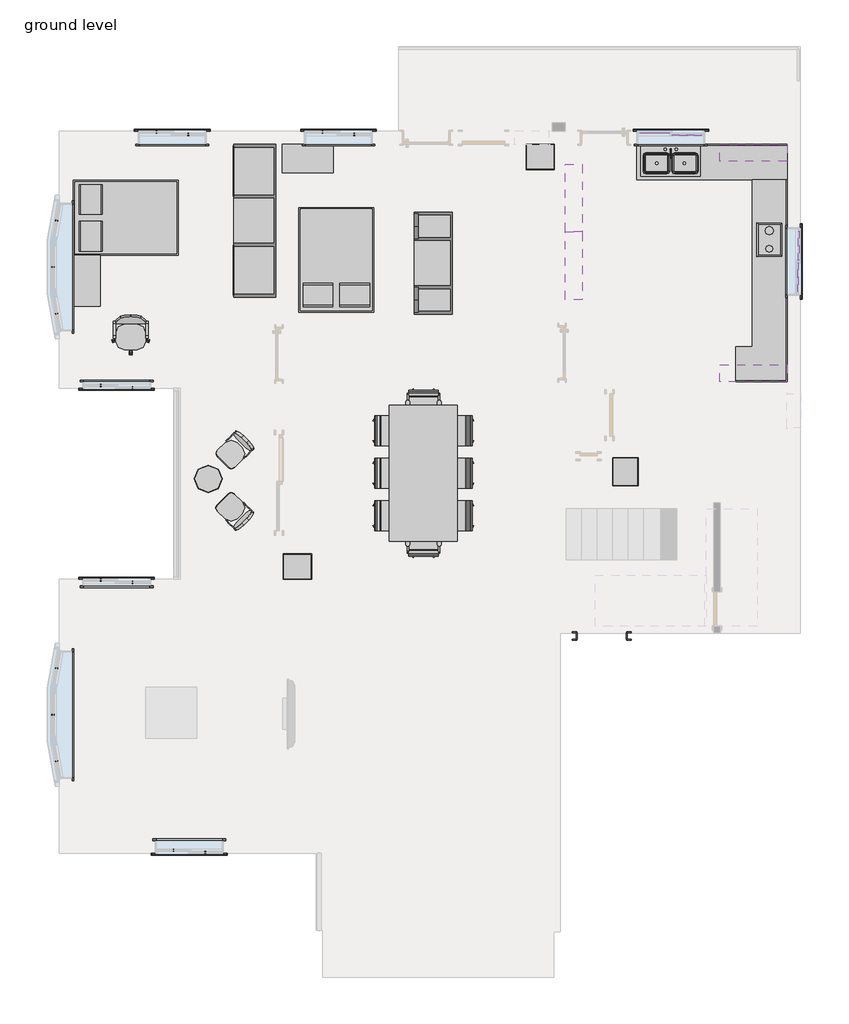
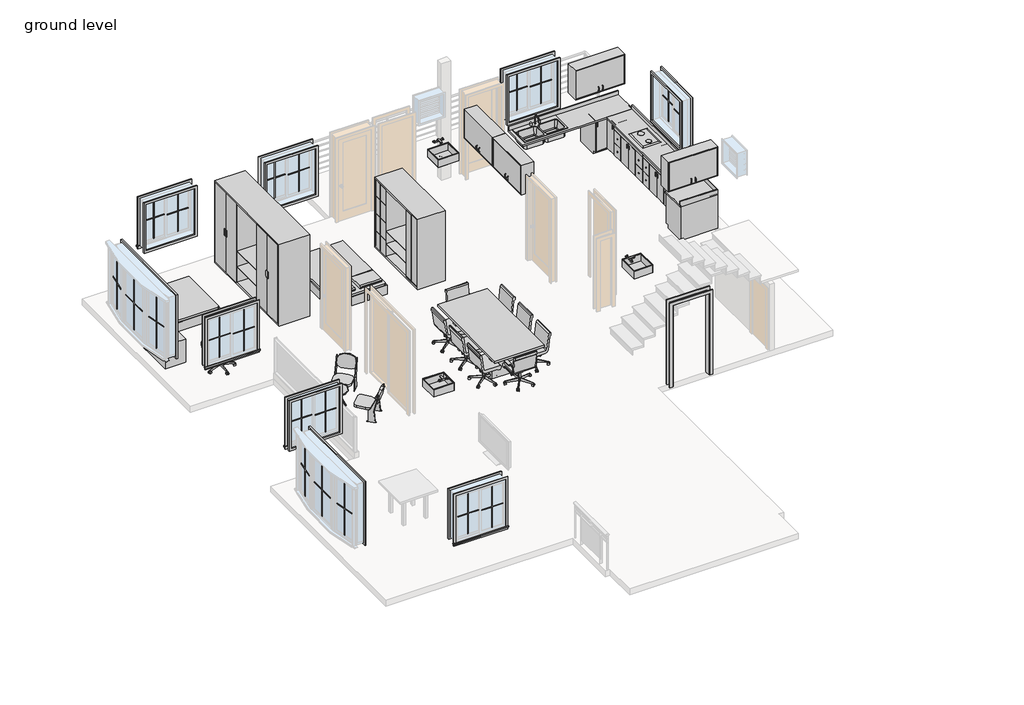
# One storey, part 2 of 2: 38 proxies, 29 furniture elements, 4 flow terminals.
"""IFC4 building model written with IfcOpenShell, lengths in millimetres."""

from ifc_helpers import new_model, si_unit, origin, place, context, project, spatial, transform, mapped, element, save
from components import proxy_3c1fa1d0, muntin_pattern_2x2_muntin_pattern_2x2_d8607f27, muntin_pattern_2x2_muntin_pattern_2x2_395d1e8c, muntin_pattern_2x2_muntin_pattern_2x2_cf37b409, proxy_99694262, trim_window_exterior_flat_with_sill_7cfdd449, trim_window_interior_flat_picture_frame_9ca7b173, trim_window_interior_flat_picture_frame_f1e0b15b, flow_terminal_cce4e9d2, flow_terminal_a53be723, furniture_e236c193, furniture_13b99e4d, furniture_b58f7881, furniture_6b884072, chair_executive_chair_executive_a6d00652, chair_task_chair_task_b7f3823b, chair_task_arms_chair_task_arms_fa5a08ef, furniture_e2cf6ce7, furniture_0681fcb1, furniture_88072bd9, furniture_1f19b6cd, furniture_eb3a3c23, furniture_6f689152, furniture_9d41381f, furniture_ea954fa4

model = new_model("IFC4")

# Units and contexts
model_context = context("Model", 3, world=origin())
ifc_project = project(units=[si_unit("LENGTHUNIT", "METRE", prefix="MILLI")], contexts=[model_context])

# Site, building, storey
site = spatial("IfcSite", under=ifc_project)
building = spatial("IfcBuilding", under=site)
storey = spatial("IfcBuildingStorey", under=building, Name="ground level", Elevation=609.6)

# Proxies
placement = place(None, origin())
proxy_shape = proxy_3c1fa1d0(model_context)
element("IfcBuildingElementProxy", 1, Name="Cook Top-2 Unit : 12\" x 18\" 2", ObjectType="Cook Top-2 Unit : 12\" x 18\" 2", at=placement, inside=storey, context=model_context, shape_type="MappedRepresentation", body=[
    mapped(proxy_shape, transform((-1317.9219122, 8623.5920118, 609.6), x_axis=(1.0, 0.0, 0.0), y_axis=(0.0, 1.0, 0.0), z_axis=(0.0, 0.0, 1.0))),
])
muntin_pattern_2x2_muntin_pattern_2x2_shape = muntin_pattern_2x2_muntin_pattern_2x2_d8607f27(model_context)
element("IfcBuildingElementProxy", 2, Name="Muntin Pattern_2x2 : Muntin Pattern_2x2", ObjectType="Muntin Pattern_2x2 : Muntin Pattern_2x2", at=placement, inside=storey, context=model_context, shape_type="MappedRepresentation", body=[
    mapped(muntin_pattern_2x2_muntin_pattern_2x2_shape, transform((-14097.2969122, 8161.6918074, 1339.85), x_axis=(0.0, 1.0, 0.0), y_axis=(-1.0, 0.0, 0.0), z_axis=(0.0, 0.0, 1.0))),
])
element("IfcBuildingElementProxy", 3, Name="Muntin Pattern_2x2 : Muntin Pattern_2x2", ObjectType="Muntin Pattern_2x2 : Muntin Pattern_2x2", at=placement, inside=storey, context=model_context, shape_type="MappedRepresentation", body=[
    mapped(muntin_pattern_2x2_muntin_pattern_2x2_shape, transform((-14097.2969122, 128.9418074, 1339.85), x_axis=(0.0, 1.0, 0.0), y_axis=(-1.0, 0.0, 0.0), z_axis=(0.0, 0.0, 1.0))),
])
muntin_pattern_2x2_muntin_pattern_2x2_2_shape = muntin_pattern_2x2_muntin_pattern_2x2_395d1e8c(model_context)
element("IfcBuildingElementProxy", 4, Name="Muntin Pattern_2x2 : Muntin Pattern_2x2", ObjectType="Muntin Pattern_2x2 : Muntin Pattern_2x2", at=placement, inside=storey, context=model_context, shape_type="MappedRepresentation", body=[
    mapped(muntin_pattern_2x2_muntin_pattern_2x2_2_shape, transform((-14032.7059546, 7325.3224399, 1339.85), x_axis=(-0.1736481776669241, 0.9848077530122091, 0.0), y_axis=(-0.9848077530122091, -0.1736481776669241, 0.0), z_axis=(0.0, 0.0, 1.0))),
])
element("IfcBuildingElementProxy", 5, Name="Muntin Pattern_2x2 : Muntin Pattern_2x2", ObjectType="Muntin Pattern_2x2 : Muntin Pattern_2x2", at=placement, inside=storey, context=model_context, shape_type="MappedRepresentation", body=[
    mapped(muntin_pattern_2x2_muntin_pattern_2x2_2_shape, transform((-14032.7059546, 8998.0611749, 1339.85), x_axis=(0.17364817766693658, 0.984807753012207, 0.0), y_axis=(-0.984807753012207, 0.17364817766693658, 0.0), z_axis=(0.0, 0.0, 1.0))),
])
element("IfcBuildingElementProxy", 6, Name="Muntin Pattern_2x2 : Muntin Pattern_2x2", ObjectType="Muntin Pattern_2x2 : Muntin Pattern_2x2", at=placement, inside=storey, context=model_context, shape_type="MappedRepresentation", body=[
    mapped(muntin_pattern_2x2_muntin_pattern_2x2_2_shape, transform((-14032.7059546, -707.4275601, 1339.85), x_axis=(-0.1736481776669241, 0.9848077530122091, 0.0), y_axis=(-0.9848077530122091, -0.1736481776669241, 0.0), z_axis=(0.0, 0.0, 1.0))),
])
element("IfcBuildingElementProxy", 7, Name="Muntin Pattern_2x2 : Muntin Pattern_2x2", ObjectType="Muntin Pattern_2x2 : Muntin Pattern_2x2", at=placement, inside=storey, context=model_context, shape_type="MappedRepresentation", body=[
    mapped(muntin_pattern_2x2_muntin_pattern_2x2_2_shape, transform((-14032.7059546, 965.3111749, 1339.85), x_axis=(0.17364817766693658, 0.984807753012207, 0.0), y_axis=(-0.984807753012207, 0.17364817766693658, 0.0), z_axis=(0.0, 0.0, 1.0))),
])
muntin_pattern_2x2_muntin_pattern_2x2_3_shape = muntin_pattern_2x2_muntin_pattern_2x2_cf37b409(model_context)
element("IfcBuildingElementProxy", 8, Name="Muntin Pattern_2x2 : Muntin Pattern_2x2", ObjectType="Muntin Pattern_2x2 : Muntin Pattern_2x2", at=placement, inside=storey, context=model_context, shape_type="MappedRepresentation", body=[
    mapped(muntin_pattern_2x2_muntin_pattern_2x2_3_shape, transform((-11936.7094122, -2303.1081926, 1606.55), x_axis=(-1.0, 0.0, 0.0), y_axis=(0.0, -1.0, 0.0), z_axis=(0.0, 0.0, 1.0))),
])
element("IfcBuildingElementProxy", 9, Name="Muntin Pattern_2x2 : Muntin Pattern_2x2", ObjectType="Muntin Pattern_2x2 : Muntin Pattern_2x2", at=placement, inside=storey, context=model_context, shape_type="MappedRepresentation", body=[
    mapped(muntin_pattern_2x2_muntin_pattern_2x2_3_shape, transform((-11368.3844122, -2347.5581926, 1606.55), x_axis=(-1.0, 0.0, 0.0), y_axis=(0.0, -1.0, 0.0), z_axis=(0.0, 0.0, 1.0))),
])
element("IfcBuildingElementProxy", 10, Name="Muntin Pattern_2x2 : Muntin Pattern_2x2", ObjectType="Muntin Pattern_2x2 : Muntin Pattern_2x2", at=placement, inside=storey, context=model_context, shape_type="MappedRepresentation", body=[
    mapped(muntin_pattern_2x2_muntin_pattern_2x2_3_shape, transform((-12673.3094122, 2503.8418074, 1606.55), x_axis=(1.0, 0.0, 0.0), y_axis=(0.0, 1.0, 0.0), z_axis=(0.0, 0.0, 1.0))),
])
element("IfcBuildingElementProxy", 11, Name="Muntin Pattern_2x2 : Muntin Pattern_2x2", ObjectType="Muntin Pattern_2x2 : Muntin Pattern_2x2", at=placement, inside=storey, context=model_context, shape_type="MappedRepresentation", body=[
    mapped(muntin_pattern_2x2_muntin_pattern_2x2_3_shape, transform((-13241.6344122, 2548.2918074, 1606.55), x_axis=(1.0, 0.0, 0.0), y_axis=(0.0, 1.0, 0.0), z_axis=(0.0, 0.0, 1.0))),
])
element("IfcBuildingElementProxy", 12, Name="Muntin Pattern_2x2 : Muntin Pattern_2x2", ObjectType="Muntin Pattern_2x2 : Muntin Pattern_2x2", at=placement, inside=storey, context=model_context, shape_type="MappedRepresentation", body=[
    mapped(muntin_pattern_2x2_muntin_pattern_2x2_3_shape, transform((-743.2469122, 7979.1293074, 1835.15), x_axis=(0.0, -1.0, 0.0), y_axis=(1.0, 0.0, 0.0), z_axis=(0.0, 0.0, 1.0))),
])
element("IfcBuildingElementProxy", 13, Name="Muntin Pattern_2x2 : Muntin Pattern_2x2", ObjectType="Muntin Pattern_2x2 : Muntin Pattern_2x2", at=placement, inside=storey, context=model_context, shape_type="MappedRepresentation", body=[
    mapped(muntin_pattern_2x2_muntin_pattern_2x2_3_shape, transform((-698.7969122, 8547.4543074, 1835.15), x_axis=(0.0, -1.0, 0.0), y_axis=(1.0, 0.0, 0.0), z_axis=(0.0, 0.0, 1.0))),
])
element("IfcBuildingElementProxy", 14, Name="Muntin Pattern_2x2 : Muntin Pattern_2x2", ObjectType="Muntin Pattern_2x2 : Muntin Pattern_2x2", at=placement, inside=storey, context=model_context, shape_type="MappedRepresentation", body=[
    mapped(muntin_pattern_2x2_muntin_pattern_2x2_3_shape, transform((-8691.8594122, 10542.9418074, 1606.55), x_axis=(1.0, 0.0, 0.0), y_axis=(0.0, 1.0, 0.0), z_axis=(0.0, 0.0, 1.0))),
])
element("IfcBuildingElementProxy", 15, Name="Muntin Pattern_2x2 : Muntin Pattern_2x2", ObjectType="Muntin Pattern_2x2 : Muntin Pattern_2x2", at=placement, inside=storey, context=model_context, shape_type="MappedRepresentation", body=[
    mapped(muntin_pattern_2x2_muntin_pattern_2x2_3_shape, transform((-9260.1844122, 10587.3918074, 1606.55), x_axis=(1.0, 0.0, 0.0), y_axis=(0.0, 1.0, 0.0), z_axis=(0.0, 0.0, 1.0))),
])
element("IfcBuildingElementProxy", 16, Name="Muntin Pattern_2x2 : Muntin Pattern_2x2", ObjectType="Muntin Pattern_2x2 : Muntin Pattern_2x2", at=placement, inside=storey, context=model_context, shape_type="MappedRepresentation", body=[
    mapped(muntin_pattern_2x2_muntin_pattern_2x2_3_shape, transform((-11673.1844122, 10542.9418074, 1606.55), x_axis=(1.0, 0.0, 0.0), y_axis=(0.0, 1.0, 0.0), z_axis=(0.0, 0.0, 1.0))),
])
element("IfcBuildingElementProxy", 17, Name="Muntin Pattern_2x2 : Muntin Pattern_2x2", ObjectType="Muntin Pattern_2x2 : Muntin Pattern_2x2", at=placement, inside=storey, context=model_context, shape_type="MappedRepresentation", body=[
    mapped(muntin_pattern_2x2_muntin_pattern_2x2_3_shape, transform((-12241.5094122, 10587.3918074, 1606.55), x_axis=(1.0, 0.0, 0.0), y_axis=(0.0, 1.0, 0.0), z_axis=(0.0, 0.0, 1.0))),
])
element("IfcBuildingElementProxy", 18, Name="Muntin Pattern_2x2 : Muntin Pattern_2x2", ObjectType="Muntin Pattern_2x2 : Muntin Pattern_2x2", at=placement, inside=storey, context=model_context, shape_type="MappedRepresentation", body=[
    mapped(muntin_pattern_2x2_muntin_pattern_2x2_3_shape, transform((-13241.6344122, 6040.7918074, 1606.55), x_axis=(-1.0, 0.0, 0.0), y_axis=(0.0, -1.0, 0.0), z_axis=(0.0, 0.0, 1.0))),
])
element("IfcBuildingElementProxy", 19, Name="Muntin Pattern_2x2 : Muntin Pattern_2x2", ObjectType="Muntin Pattern_2x2 : Muntin Pattern_2x2", at=placement, inside=storey, context=model_context, shape_type="MappedRepresentation", body=[
    mapped(muntin_pattern_2x2_muntin_pattern_2x2_3_shape, transform((-12673.3094122, 5996.3418074, 1606.55), x_axis=(-1.0, 0.0, 0.0), y_axis=(0.0, -1.0, 0.0), z_axis=(0.0, 0.0, 1.0))),
])
element("IfcBuildingElementProxy", 20, Name="Muntin Pattern_2x2 : Muntin Pattern_2x2", ObjectType="Muntin Pattern_2x2 : Muntin Pattern_2x2", at=placement, inside=storey, context=model_context, shape_type="MappedRepresentation", body=[
    mapped(muntin_pattern_2x2_muntin_pattern_2x2_3_shape, transform((-2726.0344122, 10542.9418074, 1809.75), x_axis=(1.0, 0.0, 0.0), y_axis=(0.0, 1.0, 0.0), z_axis=(0.0, 0.0, 1.0))),
])
element("IfcBuildingElementProxy", 21, Name="Muntin Pattern_2x2 : Muntin Pattern_2x2", ObjectType="Muntin Pattern_2x2 : Muntin Pattern_2x2", at=placement, inside=storey, context=model_context, shape_type="MappedRepresentation", body=[
    mapped(muntin_pattern_2x2_muntin_pattern_2x2_3_shape, transform((-3294.3594122, 10587.3918074, 1809.75), x_axis=(1.0, 0.0, 0.0), y_axis=(0.0, 1.0, 0.0), z_axis=(0.0, 0.0, 1.0))),
])
proxy_2_shape = proxy_99694262(model_context)
element("IfcBuildingElementProxy", 22, Name="Passage Opening-Cased : 36\" x 84\"", ObjectType="Passage Opening-Cased : 36\" x 84\"", at=placement, inside=storey, context=model_context, shape_type="MappedRepresentation", body=[
    mapped(proxy_2_shape, transform((-4242.6395055, 1538.6418074, 609.6), x_axis=(1.0, 0.0, 0.0), y_axis=(0.0, 1.0, 0.0), z_axis=(0.0, 0.0, 1.0))),
])
trim_window_exterior_flat_with_sill_shape = trim_window_exterior_flat_with_sill_7cfdd449(model_context)
element("IfcBuildingElementProxy", 23, Name="Trim-Window-Exterior-Flat : with Sill", ObjectType="Trim-Window-Exterior-Flat : with Sill", at=placement, inside=storey, context=model_context, shape_type="MappedRepresentation", body=[
    mapped(trim_window_exterior_flat_with_sill_shape, transform((-11652.5469122, -2357.0831926, 2743.2), x_axis=(1.0, 0.0, 0.0), y_axis=(0.0, 0.0, 1.0), z_axis=(0.0, -1.0, 0.0))),
])
element("IfcBuildingElementProxy", 24, Name="Trim-Window-Exterior-Flat : with Sill", ObjectType="Trim-Window-Exterior-Flat : with Sill", at=placement, inside=storey, context=model_context, shape_type="MappedRepresentation", body=[
    mapped(trim_window_exterior_flat_with_sill_shape, transform((-12957.4719122, 2557.8168074, 2743.2), x_axis=(-1.0, 0.0, 0.0), y_axis=(0.0, 0.0, 1.0), z_axis=(0.0, 1.0, 0.0))),
])
element("IfcBuildingElementProxy", 25, Name="Trim-Window-Exterior-Flat : with Sill", ObjectType="Trim-Window-Exterior-Flat : with Sill", at=placement, inside=storey, context=model_context, shape_type="MappedRepresentation", body=[
    mapped(trim_window_exterior_flat_with_sill_shape, transform((-689.2719122, 8263.2918074, 2971.8), x_axis=(0.0, 1.0, 0.0), y_axis=(0.0, 0.0, 1.0), z_axis=(1.0, 0.0, 0.0))),
])
element("IfcBuildingElementProxy", 26, Name="Trim-Window-Exterior-Flat : with Sill", ObjectType="Trim-Window-Exterior-Flat : with Sill", at=placement, inside=storey, context=model_context, shape_type="MappedRepresentation", body=[
    mapped(trim_window_exterior_flat_with_sill_shape, transform((-8976.0219122, 10596.9168074, 2743.2), x_axis=(-1.0, 0.0, 0.0), y_axis=(0.0, 0.0, 1.0), z_axis=(0.0, 1.0, 0.0))),
])
element("IfcBuildingElementProxy", 27, Name="Trim-Window-Exterior-Flat : with Sill", ObjectType="Trim-Window-Exterior-Flat : with Sill", at=placement, inside=storey, context=model_context, shape_type="MappedRepresentation", body=[
    mapped(trim_window_exterior_flat_with_sill_shape, transform((-11957.3469122, 10596.9168074, 2743.2), x_axis=(-1.0, 0.0, 0.0), y_axis=(0.0, 0.0, 1.0), z_axis=(0.0, 1.0, 0.0))),
])
element("IfcBuildingElementProxy", 28, Name="Trim-Window-Exterior-Flat : with Sill", ObjectType="Trim-Window-Exterior-Flat : with Sill", at=placement, inside=storey, context=model_context, shape_type="MappedRepresentation", body=[
    mapped(trim_window_exterior_flat_with_sill_shape, transform((-12957.4719122, 5986.8168074, 2743.2), x_axis=(1.0, 0.0, 0.0), y_axis=(0.0, 0.0, 1.0), z_axis=(0.0, -1.0, 0.0))),
])
element("IfcBuildingElementProxy", 29, Name="Trim-Window-Exterior-Flat : with Sill", ObjectType="Trim-Window-Exterior-Flat : with Sill", at=placement, inside=storey, context=model_context, shape_type="MappedRepresentation", body=[
    mapped(trim_window_exterior_flat_with_sill_shape, transform((-3010.1969122, 10596.9168074, 2946.4), x_axis=(-1.0, 0.0, 0.0), y_axis=(0.0, 0.0, 1.0), z_axis=(0.0, 1.0, 0.0))),
])
trim_window_interior_flat_picture_frame_shape = trim_window_interior_flat_picture_frame_9ca7b173(model_context)
element("IfcBuildingElementProxy", 30, Name="Trim-Window-Interior-Flat : Picture Frame", ObjectType="Trim-Window-Interior-Flat : Picture Frame", at=placement, inside=storey, context=model_context, shape_type="MappedRepresentation", body=[
    mapped(trim_window_interior_flat_picture_frame_shape, transform((-13757.5719122, 8161.6918074, 2794.0), x_axis=(0.0, 1.0, 0.0), y_axis=(0.0, 0.0, 1.0), z_axis=(1.0, 0.0, 0.0))),
])
element("IfcBuildingElementProxy", 31, Name="Trim-Window-Interior-Flat : Picture Frame", ObjectType="Trim-Window-Interior-Flat : Picture Frame", at=placement, inside=storey, context=model_context, shape_type="MappedRepresentation", body=[
    mapped(trim_window_interior_flat_picture_frame_shape, transform((-13757.5719122, 128.9418074, 2794.0), x_axis=(0.0, 1.0, 0.0), y_axis=(0.0, 0.0, 1.0), z_axis=(1.0, 0.0, 0.0))),
])
trim_window_interior_flat_picture_frame_2_shape = trim_window_interior_flat_picture_frame_f1e0b15b(model_context)
element("IfcBuildingElementProxy", 32, Name="Trim-Window-Interior-Flat : Picture Frame", ObjectType="Trim-Window-Interior-Flat : Picture Frame", at=placement, inside=storey, context=model_context, shape_type="MappedRepresentation", body=[
    mapped(trim_window_interior_flat_picture_frame_2_shape, transform((-11652.5469122, -2128.4831926, 2743.2), x_axis=(-1.0, 0.0, 0.0), y_axis=(0.0, 0.0, 1.0), z_axis=(0.0, 1.0, 0.0))),
])
element("IfcBuildingElementProxy", 33, Name="Trim-Window-Interior-Flat : Picture Frame", ObjectType="Trim-Window-Interior-Flat : Picture Frame", at=placement, inside=storey, context=model_context, shape_type="MappedRepresentation", body=[
    mapped(trim_window_interior_flat_picture_frame_2_shape, transform((-12957.4719122, 2443.5168074, 2743.2), x_axis=(1.0, 0.0, 0.0), y_axis=(0.0, 0.0, 1.0), z_axis=(0.0, -1.0, 0.0))),
])
element("IfcBuildingElementProxy", 34, Name="Trim-Window-Interior-Flat : Picture Frame", ObjectType="Trim-Window-Interior-Flat : Picture Frame", at=placement, inside=storey, context=model_context, shape_type="MappedRepresentation", body=[
    mapped(trim_window_interior_flat_picture_frame_2_shape, transform((-917.8719122, 8263.2918074, 2971.8), x_axis=(0.0, -1.0, 0.0), y_axis=(0.0, 0.0, 1.0), z_axis=(-1.0, 0.0, 0.0))),
])
element("IfcBuildingElementProxy", 35, Name="Trim-Window-Interior-Flat : Picture Frame", ObjectType="Trim-Window-Interior-Flat : Picture Frame", at=placement, inside=storey, context=model_context, shape_type="MappedRepresentation", body=[
    mapped(trim_window_interior_flat_picture_frame_2_shape, transform((-8976.0219122, 10368.3168074, 2743.2), x_axis=(1.0, 0.0, 0.0), y_axis=(0.0, 0.0, 1.0), z_axis=(0.0, -1.0, 0.0))),
])
element("IfcBuildingElementProxy", 36, Name="Trim-Window-Interior-Flat : Picture Frame", ObjectType="Trim-Window-Interior-Flat : Picture Frame", at=placement, inside=storey, context=model_context, shape_type="MappedRepresentation", body=[
    mapped(trim_window_interior_flat_picture_frame_2_shape, transform((-11957.3469122, 10368.3168074, 2743.2), x_axis=(1.0, 0.0, 0.0), y_axis=(0.0, 0.0, 1.0), z_axis=(0.0, -1.0, 0.0))),
])
element("IfcBuildingElementProxy", 37, Name="Trim-Window-Interior-Flat : Picture Frame", ObjectType="Trim-Window-Interior-Flat : Picture Frame", at=placement, inside=storey, context=model_context, shape_type="MappedRepresentation", body=[
    mapped(trim_window_interior_flat_picture_frame_2_shape, transform((-12957.4719122, 6101.1168074, 2743.2), x_axis=(-1.0, 0.0, 0.0), y_axis=(0.0, 0.0, 1.0), z_axis=(0.0, 1.0, 0.0))),
])
element("IfcBuildingElementProxy", 38, Name="Trim-Window-Interior-Flat : Picture Frame", ObjectType="Trim-Window-Interior-Flat : Picture Frame", at=placement, inside=storey, context=model_context, shape_type="MappedRepresentation", body=[
    mapped(trim_window_interior_flat_picture_frame_2_shape, transform((-3010.1969122, 10368.3168074, 2946.4), x_axis=(1.0, 0.0, 0.0), y_axis=(0.0, 0.0, 1.0), z_axis=(0.0, -1.0, 0.0))),
])

# Flow terminals
flow_terminal_shape = flow_terminal_cce4e9d2(model_context)
element("IfcFlowTerminal", 39, ObjectType="Sink - Work : 20\"x18\"", at=placement, inside=storey, context=model_context, shape_type="MappedRepresentation", body=[
    mapped(flow_terminal_shape, transform((-5353.3469122, 10368.3168074, 1524.0), x_axis=(1.0, 0.0, 0.0), y_axis=(0.0, 1.0, 0.0), z_axis=(0.0, 0.0, 1.0))),
])
element("IfcFlowTerminal", 40, ObjectType="Sink - Work : 20\"x18\"", at=placement, inside=storey, context=model_context, shape_type="MappedRepresentation", body=[
    mapped(flow_terminal_shape, transform((-4054.7719122, 4488.2168074, 1524.0), x_axis=(0.0, 1.0, 0.0), y_axis=(-1.0, 0.0, 0.0), z_axis=(0.0, 0.0, 1.0))),
])
element("IfcFlowTerminal", 41, ObjectType="Sink - Work : 20\"x18\"", at=placement, inside=storey, context=model_context, shape_type="MappedRepresentation", body=[
    mapped(flow_terminal_shape, transform((-9712.6219122, 2557.8168074, 1524.0), x_axis=(-1.0, 0.0, 0.0), y_axis=(0.0, -1.0, 0.0), z_axis=(0.0, 0.0, 1.0))),
])
flow_terminal_2_shape = flow_terminal_a53be723(model_context)
element("IfcFlowTerminal", 42, ObjectType="Sink Kitchen-Double : 42\" x 21\"", at=placement, inside=storey, context=model_context, shape_type="MappedRepresentation", body=[
    mapped(flow_terminal_2_shape, transform((-3029.0611528, 10061.1714063, 609.6), x_axis=(1.0, 0.0, 0.0), y_axis=(0.0, 1.0, 0.0), z_axis=(0.0, 0.0, 1.0))),
])

# Furniture
furniture_shape = furniture_e236c193(model_context)
element("IfcFurniture", 43, ObjectType="48\" 2", at=placement, inside=storey, context=model_context, shape_type="MappedRepresentation", body=[
    mapped(furniture_shape, transform((-917.8719122, 8935.1617674, 609.6), x_axis=(0.0, -1.0, 0.0), y_axis=(1.0, 0.0, 0.0), z_axis=(0.0, 0.0, 1.0))),
])
element("IfcFurniture", 44, ObjectType="48\" 2", at=placement, inside=storey, context=model_context, shape_type="MappedRepresentation", body=[
    mapped(furniture_shape, transform((-917.8719122, 7715.9617674, 609.6), x_axis=(0.0, -1.0, 0.0), y_axis=(1.0, 0.0, 0.0), z_axis=(0.0, 0.0, 1.0))),
])
furniture_2_shape = furniture_13b99e4d(model_context)
element("IfcFurniture", 45, ObjectType="Base Cabinet-Corner Unit-Square : 36\" 2", at=placement, inside=storey, context=model_context, shape_type="MappedRepresentation", body=[
    mapped(furniture_2_shape, transform((-1444.6096171, 10368.3168074, 609.6), x_axis=(1.0, 0.0, 0.0), y_axis=(0.0, 1.0, 0.0), z_axis=(0.0, 0.0, 1.0))),
])
element("IfcFurniture", 46, ObjectType="Base Cabinet-Corner Unit-Square : 36\" 2", at=placement, inside=storey, context=model_context, shape_type="MappedRepresentation", body=[
    mapped(furniture_2_shape, transform((-917.8719122, 6627.8545123, 609.6), x_axis=(0.0, -1.0, 0.0), y_axis=(1.0, 0.0, 0.0), z_axis=(0.0, 0.0, 1.0))),
])
furniture_3_shape = furniture_b58f7881(model_context)
element("IfcFurniture", 47, ObjectType="Bed-Box : Double 53\" x 74\"", at=placement, inside=storey, context=model_context, shape_type="MappedRepresentation", body=[
    mapped(furniture_3_shape, transform((-13026.8014204, 8708.3643484, 609.6), x_axis=(0.0, 1.0, 0.0), y_axis=(-1.0, 0.0, 0.0), z_axis=(0.0, 0.0, 1.0))),
])
element("IfcFurniture", 48, ObjectType="Bed-Box : Double 53\" x 74\"", at=placement, inside=storey, context=model_context, shape_type="MappedRepresentation", body=[
    mapped(furniture_3_shape, transform((-8674.9694532, 8057.4372992, 609.6), x_axis=(-1.0, 0.0, 0.0), y_axis=(0.0, -1.0, 0.0), z_axis=(0.0, 0.0, 1.0))),
])
furniture_4_shape = furniture_6b884072(model_context)
element("IfcFurniture", 49, ObjectType="Cabinet File-Lateral 2 Drawer : 36\" x 20\" x 24\"", at=placement, inside=storey, context=model_context, shape_type="MappedRepresentation", body=[
    mapped(furniture_4_shape, transform((-14437.8902883, 8097.2393213, 609.6), x_axis=(0.0, 1.0, 0.0), y_axis=(-1.0, 0.0, 0.0), z_axis=(0.0, 0.0, 1.0))),
])
element("IfcFurniture", 50, ObjectType="Cabinet File-Lateral 2 Drawer : 36\" x 20\" x 24\"", at=placement, inside=storey, context=model_context, shape_type="MappedRepresentation", body=[
    mapped(furniture_4_shape, transform((-9348.4493983, 11048.6351835, 609.6), x_axis=(1.0, 0.0, 0.0), y_axis=(0.0, 1.0, 0.0), z_axis=(0.0, 0.0, 1.0))),
])
chair_executive_chair_executive_shape = chair_executive_chair_executive_a6d00652(model_context)
element("IfcFurniture", 51, ObjectType="Chair-Executive : Chair-Executive", at=placement, inside=storey, context=model_context, shape_type="MappedRepresentation", body=[
    mapped(chair_executive_chair_executive_shape, transform((-12562.4810925, 6958.262709, 609.6), x_axis=(-1.0, 0.0, 0.0), y_axis=(0.0, -1.0, 0.0), z_axis=(0.0, 0.0, 1.0))),
])
chair_task_chair_task_shape = chair_task_chair_task_b7f3823b(model_context)
element("IfcFurniture", 52, ObjectType="Chair-Task : Chair-Task", at=placement, inside=storey, context=model_context, shape_type="MappedRepresentation", body=[
    mapped(chair_task_chair_task_shape, transform((-8080.5678138, 4603.8076271, 609.6), x_axis=(0.0, -1.0, 0.0), y_axis=(1.0, 0.0, 0.0), z_axis=(0.0, 0.0, 1.0))),
])
element("IfcFurniture", 53, ObjectType="Chair-Task : Chair-Task", at=placement, inside=storey, context=model_context, shape_type="MappedRepresentation", body=[
    mapped(chair_task_chair_task_shape, transform((-8080.5678138, 5365.8076271, 609.6), x_axis=(0.0, -1.0, 0.0), y_axis=(1.0, 0.0, 0.0), z_axis=(0.0, 0.0, 1.0))),
])
element("IfcFurniture", 54, ObjectType="Chair-Task : Chair-Task", at=placement, inside=storey, context=model_context, shape_type="MappedRepresentation", body=[
    mapped(chair_task_chair_task_shape, transform((-6823.4760106, 4321.8259877, 609.6), x_axis=(0.0, 1.0, 0.0), y_axis=(-1.0, 0.0, 0.0), z_axis=(0.0, 0.0, 1.0))),
])
element("IfcFurniture", 55, ObjectType="Chair-Task : Chair-Task", at=placement, inside=storey, context=model_context, shape_type="MappedRepresentation", body=[
    mapped(chair_task_chair_task_shape, transform((-6823.4760106, 5083.8259877, 609.6), x_axis=(0.0, 1.0, 0.0), y_axis=(-1.0, 0.0, 0.0), z_axis=(0.0, 0.0, 1.0))),
])
element("IfcFurniture", 56, ObjectType="Chair-Task : Chair-Task", at=placement, inside=storey, context=model_context, shape_type="MappedRepresentation", body=[
    mapped(chair_task_chair_task_shape, transform((-8080.5678138, 3841.8076271, 609.6), x_axis=(0.0, -1.0, 0.0), y_axis=(1.0, 0.0, 0.0), z_axis=(0.0, 0.0, 1.0))),
])
element("IfcFurniture", 57, ObjectType="Chair-Task : Chair-Task", at=placement, inside=storey, context=model_context, shape_type="MappedRepresentation", body=[
    mapped(chair_task_chair_task_shape, transform((-6823.4760106, 3559.8259877, 609.6), x_axis=(0.0, 1.0, 0.0), y_axis=(-1.0, 0.0, 0.0), z_axis=(0.0, 0.0, 1.0))),
])
chair_task_arms_chair_task_arms_shape = chair_task_arms_chair_task_arms_fa5a08ef(model_context)
element("IfcFurniture", 58, ObjectType="Chair-Task Arms : Chair-Task Arms", at=placement, inside=storey, context=model_context, shape_type="MappedRepresentation", body=[
    mapped(chair_task_arms_chair_task_arms_shape, transform((-7593.0127319, 3224.6709058, 609.6), x_axis=(1.0, 0.0, 0.0), y_axis=(0.0, 1.0, 0.0), z_axis=(0.0, 0.0, 1.0))),
])
element("IfcFurniture", 59, ObjectType="Chair-Task Arms : Chair-Task Arms", at=placement, inside=storey, context=model_context, shape_type="MappedRepresentation", body=[
    mapped(chair_task_arms_chair_task_arms_shape, transform((-7311.0310925, 5700.962709, 609.6), x_axis=(-1.0, 0.0, 0.0), y_axis=(0.0, -1.0, 0.0), z_axis=(0.0, 0.0, 1.0))),
])
furniture_5_shape = furniture_e2cf6ce7(model_context)
element("IfcFurniture", 60, ObjectType="Counter Top w Sink : 24\" Depth", at=placement, inside=storey, context=model_context, shape_type="MappedRepresentation", body=[
    mapped(furniture_5_shape, transform((-2422.5096171, 10368.3168074, 609.6), x_axis=(1.0, 0.0, 0.0), y_axis=(0.0, 1.0, 0.0), z_axis=(0.0, 0.0, 1.0))),
])
furniture_6_shape = furniture_0681fcb1(model_context)
element("IfcFurniture", 61, ObjectType="Counter Top-L Shaped : 24\" Depth", at=placement, inside=storey, context=model_context, shape_type="MappedRepresentation", body=[
    mapped(furniture_6_shape, transform((-2118.3342073, 6101.1168074, 609.6), x_axis=(-1.0, 0.0, 0.0), y_axis=(0.0, -1.0, 0.0), z_axis=(0.0, 0.0, 1.0))),
])
furniture_7_shape = furniture_88072bd9(model_context)
element("IfcFurniture", 62, ObjectType="Entertainment Center.0001 : 72\" x 72\" x 24\"", at=placement, inside=storey, context=model_context, shape_type="MappedRepresentation", body=[
    mapped(furniture_7_shape, transform((-6836.0719122, 8234.7168074, 609.6), x_axis=(0.0, -1.0, 0.0), y_axis=(1.0, 0.0, 0.0), z_axis=(0.0, 0.0, 1.0))),
])
furniture_8_shape = furniture_1f19b6cd(model_context)
element("IfcFurniture", 63, ObjectType="Entertainment Center.0001 : 96\" x 84\" x 30\"", at=placement, inside=storey, context=model_context, shape_type="MappedRepresentation", body=[
    mapped(furniture_8_shape, transform((-10074.5719122, 8996.7168074, 609.6), x_axis=(0.0, -1.0, 0.0), y_axis=(1.0, 0.0, 0.0), z_axis=(0.0, 0.0, 1.0))),
])
furniture_9_shape = furniture_eb3a3c23(model_context)
element("IfcFurniture", 64, ObjectType="Seating-Auditorium : 18\" x 24\" x 30\"", at=placement, inside=storey, context=model_context, shape_type="MappedRepresentation", body=[
    mapped(furniture_9_shape, transform((-10585.3785026, 4901.853744, 609.6), x_axis=(-0.7071067811865437, 0.7071067811865515, 0.0), y_axis=(-0.7071067811865515, -0.7071067811865437, 0.0), z_axis=(0.0, 0.0, 1.0))),
])
element("IfcFurniture", 65, ObjectType="Seating-Auditorium : 18\" x 24\" x 30\"", at=placement, inside=storey, context=model_context, shape_type="MappedRepresentation", body=[
    mapped(furniture_9_shape, transform((-10817.6383246, 3529.1028515, 609.6), x_axis=(0.7071067811865485, 0.7071067811865466, 0.0), y_axis=(-0.7071067811865466, 0.7071067811865485, 0.0), z_axis=(0.0, 0.0, 1.0))),
])
furniture_10_shape = furniture_6f689152(model_context)
element("IfcFurniture", 66, ObjectType="Table-Conference2 w Chairs : 48\" x 144\" 2", at=placement, inside=storey, context=model_context, shape_type="MappedRepresentation", body=[
    mapped(furniture_10_shape, transform((-7452.0219122, 4462.8168074, 609.6), x_axis=(0.0, 1.0, 0.0), y_axis=(-1.0, 0.0, 0.0), z_axis=(0.0, 0.0, 1.0))),
])
furniture_11_shape = furniture_9d41381f(model_context)
element("IfcFurniture", 67, ObjectType="Table-Trio End : 20\" Diameter", at=placement, inside=storey, context=model_context, shape_type="MappedRepresentation", body=[
    mapped(furniture_11_shape, transform((-11312.8219122, 4360.062262, 609.6), x_axis=(1.0, 0.0, 0.0), y_axis=(0.0, 1.0, 0.0), z_axis=(0.0, 0.0, 1.0))),
])
furniture_12_shape = furniture_ea954fa4(model_context)
element("IfcFurniture", 68, ObjectType="Upper Cabinet-Pass-Thru : 48\" x 30\" x 12\"", at=placement, inside=storey, context=model_context, shape_type="MappedRepresentation", body=[
    mapped(furniture_12_shape, transform((-1546.2096171, 10368.3168074, 609.6), x_axis=(1.0, 0.0, 0.0), y_axis=(0.0, 1.0, 0.0), z_axis=(0.0, 0.0, 1.0))),
])
element("IfcFurniture", 69, ObjectType="Upper Cabinet-Pass-Thru : 48\" x 30\" x 12\"", at=placement, inside=storey, context=model_context, shape_type="MappedRepresentation", body=[
    mapped(furniture_12_shape, transform((-1508.7342073, 6101.1168074, 609.6), x_axis=(-1.0, 0.0, 0.0), y_axis=(0.0, -1.0, 0.0), z_axis=(0.0, 0.0, 1.0))),
])
element("IfcFurniture", 70, ObjectType="Upper Cabinet-Pass-Thru : 48\" x 30\" x 12\"", at=placement, inside=storey, context=model_context, shape_type="MappedRepresentation", body=[
    mapped(furniture_12_shape, transform((-4908.8469122, 9384.3791025, 609.6), x_axis=(0.0, 1.0, 0.0), y_axis=(-1.0, 0.0, 0.0), z_axis=(0.0, 0.0, 1.0))),
])
element("IfcFurniture", 71, ObjectType="Upper Cabinet-Pass-Thru : 48\" x 30\" x 12\"", at=placement, inside=storey, context=model_context, shape_type="MappedRepresentation", body=[
    mapped(furniture_12_shape, transform((-4908.8469122, 8165.1791025, 609.6), x_axis=(0.0, 1.0, 0.0), y_axis=(-1.0, 0.0, 0.0), z_axis=(0.0, 0.0, 1.0))),
])

save(model, "model.ifc")

# Revit data of these elements
# Type "Cook Top-2 Unit : 12\" x 18\" 2"
#   Assembly Code = "E1090400"
#   Counter Height = 3' - 0"
#   Depth = 2' - 0"
#   Width = 1' - 6"
#   Burner Material = Metal - Chrome
#   Cooktop Material = Metal - Steel, Polished
#   Default Elevation = 0
# Type "Muntin Pattern_2x2 : Muntin Pattern_2x2"
#   Width [instance default] = 4' - 0"
#   Thickness = 0' - 0 1/2"
#   Height [instance default] = 4' - 0"
#   Distance = 0' - 0 3/4"
#   Interior Material [instance default] = none
#   Exterior Material [instance default] = none
#   Default Elevation = 0
# Type "Passage Opening-Cased : 36\" x 84\""
#   Height = 7' - 0"
#   Trim Thickness = 0' - 0 3/4"
#   Trim Width = 0' - 3"
#   Width = 3' - 0"
#   Frame Material = Door - Frame
#   Default Elevation = 0
# Type "Trim-Window-Exterior-Flat : with Sill"
#   Trim Width = 0' - 2 1/4"
#   Trim Thickness_Picture Frame = 0' - 1 1/4"
#   Trim Thickness_with Sill = 0' - 0 3/4"
#   Sill Thickness = 0' - 1 1/4"
#   Opening Width [instance default] = 2' - 0"
#   Opening Height [instance default] = 3' - 0"
#   Default Elevation = 4' - 0"
#   Sill = yes
#   Picture Frame = no
#   Trim Material [instance default] = none
# Type "Trim-Window-Interior-Flat : Picture Frame"
#   Trim Thickness_Picture Frame = 0' - 1 1/4"
#   Trim Width = 0' - 2 1/4"
#   Trim Thickness_with Sill = 0' - 0 3/4"
#   Sill Thickness = 0' - 1 1/4"
#   Opening Width [instance default] = 2' - 0"
#   Opening Height [instance default] = 3' - 0"
#   Default Elevation = 4' - 0"
#   Sill = no
#   Picture Frame = yes
#   Trim Material [instance default] = none
# Type "Sink - Work : 20\"x18\""
#   WFU = 2
#   Sink Width = 1' - 6"
#   Sink Length = 1' - 8"
#   Sink Depth = 0' - 8"
#   Sanitary Radius = 3/4"
#   Sanitary Diameter = 1 1/2"
#   Hot Water Radius = 1/4"
#   Hot Water Diameter = 1/2"
#   HWFU = 2.25
#   Flow Pressure [instance default] = 8.00 psi
#   Faucet Height = 1' - 1 5/8"
#   Cold Water Radius = 1/4"
#   Cold Water Diameter = 1/2"
#   CWFU = 2.25
#   Sink Material = none
#   Faucet Material = none
#   Default Elevation = 0
# Type "Sink Kitchen-Double : 42\" x 21\""
#   Assembly Code = "D2010410"
#   Counter Height = 3' - 0"
#   Depth = 1' - 9"
#   Width = 3' - 6"
#   Faucet Material = Steel, Polished
#   Sink Material = Steel, Polished
#   Default Elevation = 0
# Type "48\" 2"
#   Assembly Code = "C1030410"
#   Depth = 2' - 0"
#   Height = 2' - 11 3/4"
#   Toe Depth = 0' - 3"
#   Toe Height = 0' - 3 1/2"
#   Width = 4' - 0"
#   Cabinet Material = none
#   Door/Drawer Material = none
#   Handle Material = Cabinets - Handles
#   Default Elevation = 0
# Type "Base Cabinet-Corner Unit-Square : 36\" 2"
#   Assembly Code = "C1030410"
#   Depth = 2' - 0"
#   Height = 2' - 11 3/4"
#   Toe Depth = 0' - 3"
#   Toe Height = 0' - 3 1/2"
#   Width = 3' - 0"
#   Cabinet Material = Cabinets
#   Door/Drawer Material = Cabinets
#   Handle Material = Cabinets - Handles
#   Default Elevation = 0
# Type "Bed-Box : Double 53\" x 74\""
#   Assembly Code = "E2020200"
#   Length = 6' - 2"
#   Width = 4' - 5"
#   Frame Material = Birch
#   Mattress Material = Linen, White
#   Default Elevation = 0
# Type "Cabinet File-Lateral 2 Drawer : 36\" x 20\" x 24\""
#   Assembly Code = "E2020200"
#   Depth = 1' - 8"
#   Height = 2' - 0"
#   Width = 3' - 0"
#   Material = Metal - Steel
#   Default Elevation = 0
# Type "Chair-Executive : Chair-Executive"
#   Assembly Code = "E2020200"
#   Base/Arms Material = Plastic, Opaque Black
#   Casters Material = Plastic, Opaque Black
#   Seat/Back Material = Textile - Slate Blue
#   Default Elevation = 0
# Type "Chair-Task : Chair-Task"
#   Assembly Code = "E2020200"
#   Base Material = Plastic - Black
#   Caster Material = Plastic - Black
#   Seat/Back Material = Textile - Slate Blue
#   Default Elevation = 0
# Type "Chair-Task Arms : Chair-Task Arms"
#   Assembly Code = "E2020200"
#   Base Material = Plastic - Black
#   Caster Material = Plastic - Black
#   Seat/Back Material = Textile - Slate Blue
#   Default Elevation = 0
# Type "Counter Top w Sink : 24\" Depth"
#   Assembly Code = "C1030400"
#   Counter Thickness = 0' - 1 1/2"
#   Depth = 2' - 1"
#   Height = 3' - 0"
#   Length [instance default] = 8' - 0"
#   Sink Location [instance default] = 2' - 0"
#   Sink Location To Wall [instance default] = 0' - 6"
#   Sink Opening Depth [instance default] = 1' - 3"
#   Sink Opening Width [instance default] = 3' - 3"
#   Counter Top Material = none
#   Default Elevation = 0
# Type "Counter Top-L Shaped : 24\" Depth"
#   Assembly Code = "C1030400"
#   Counter Thickness = 0' - 1 1/2"
#   Depth = 2' - 1"
#   Height = 3' - 0"
#   Length - Leg 1 [instance default] = 8' - 0"
#   Length - Leg 2 [instance default] = 6' - 0"
#   Counter Top Material = none
#   Default Elevation = 0
# Type "Entertainment Center.0001 : 72\" x 72\" x 24\""
#   Assembly Code = "E2020200"
#   Center Width = 2' - 8"
#   Depth = 2' - 0"
#   Height = 6' - 0"
#   Width = 6' - 0"
#   Material = none
#   Default Elevation = 0
# Type "Entertainment Center.0001 : 96\" x 84\" x 30\""
#   Assembly Code = "E2020200"
#   Center Width = 2' - 8"
#   Depth = 2' - 6"
#   Height = 7' - 0"
#   Width = 9' - 0"
#   Material = Laminate, Ivory, Matte
#   Default Elevation = 0
# Type "Seating-Auditorium : 18\" x 24\" x 30\""
#   Assembly Code = "E2020200"
#   Seat Material = Linen, Beige
#   Frame Material = Steel, Paint Finish, Dark Gray, Matte
#   Default Elevation = 0
# Type "Table-Conference2 w Chairs : 48\" x 144\" 2"
#   Assembly Code = "E2020200"
#   Description = "Seating 12-14"
#   Height = 2' - 6"
#   Length = 8' - 0"
#   Width = 4' - 0"
#   Number Of Chairs One Side = 3
#   Number Of Chairs = 8
#   Material = Wood - Cherry
#   Default Elevation = 0
# Type "Table-Trio End : 20\" Diameter"
#   Assembly Code = "E2020200"
#   Default Elevation = 0' - 6"
#   Base and Trim Material = Wood - Birch
#   Table Top Material = Laminate - Ivory,Matte
# Type "Upper Cabinet-Pass-Thru : 48\" x 30\" x 12\""
#   Depth = 1' - 0"
#   Height = 2' - 6"
#   Top of Cabinet = 7' - 0"
#   Width = 4' - 0"
#   Default Elevation = 0
# Element 1 (IfcBuildingElementProxy, "Cook Top-2 Unit : 12\" x 18\" 2")
#   Phase Created = New Construction
#   Materials on its faces: "Metal - Steel, Polished", "Metal - Chrome"
# Elements 2, 3 (IfcBuildingElementProxy, "Muntin Pattern_2x2 : Muntin Pattern_2x2")
#   Width = 2' - 3.57789"
#   Height = 4' - 6 1/2"
#   Interior Material = Wood - Stained
#   Exterior Material = Clad - White
#   Phase Created = New Construction
#   Materials on its faces: "Clad - White", "Wood - Stained"
# Elements 4, 5, 6, 7 (IfcBuildingElementProxy, "Muntin Pattern_2x2 : Muntin Pattern_2x2")
#   Width = 1' - 7.85416"
#   Height = 4' - 6 1/2"
#   Interior Material = Wood - Stained
#   Exterior Material = Clad - White
#   Phase Created = New Construction
#   Materials on its faces: "Clad - White", "Wood - Stained"
# Elements 8, 9, 10, 11, 12, 13, 14, 15, 16, 17, 18, 19, 20, 21 (IfcBuildingElementProxy, "Muntin Pattern_2x2 : Muntin Pattern_2x2")
#   Width = 1' - 8 5/8"
#   Height = 3' - 6 1/4"
#   Interior Material = Wood - Stained
#   Exterior Material = Clad - White
#   Phase Created = New Construction
#   Materials on its faces: "Clad - White", "Wood - Stained"
# Element 22 (IfcBuildingElementProxy, "Passage Opening-Cased : 36\" x 84\"")
#   Phase Created = New Construction
#   Materials on its faces: "Door - Frame"
# Elements 23, 24, 25, 26, 27, 28, 29 (IfcBuildingElementProxy, "Trim-Window-Exterior-Flat : with Sill")
#   Opening Width = 4' - 0"
#   Opening Height = 4' - 0"
#   Trim Material = Clad - White
#   Phase Created = New Construction
#   Materials on its faces: "Clad - White"
# Elements 30, 31 (IfcBuildingElementProxy, "Trim-Window-Interior-Flat : Picture Frame")
#   Opening Width = 7' - 6"
#   Opening Height = 5' - 2"
#   Trim Material = Wood - Stained
#   Phase Created = New Construction
#   Materials on its faces: "Wood - Stained"
# Elements 32, 33, 34, 35, 36, 37, 38 (IfcBuildingElementProxy, "Trim-Window-Interior-Flat : Picture Frame")
#   Opening Width = 4' - 0"
#   Opening Height = 4' - 0"
#   Trim Material = Wood - Stained
#   Phase Created = New Construction
#   Materials on its faces: "Wood - Stained"
# Element 39 (IfcFlowTerminal, "Sink - Work : 20\"x18\"")
#   Mark = "2"
#   Flow Pressure = 8.00 psi
#   Phase Created = New Construction
# Element 40 (IfcFlowTerminal, "Sink - Work : 20\"x18\"")
#   Mark = "3"
#   Flow Pressure = 8.00 psi
#   Phase Created = New Construction
# Element 41 (IfcFlowTerminal, "Sink - Work : 20\"x18\"")
#   Mark = "4"
#   Flow Pressure = 8.00 psi
#   Phase Created = New Construction
# Element 42 (IfcFlowTerminal, "Sink Kitchen-Double : 42\" x 21\"")
#   Mark = "1"
#   Phase Created = New Construction
#   Materials on its faces: "Steel, Polished"
# Elements 43, 44 (IfcFurniture, "48\" 2")
#   Phase Created = New Construction
#   Materials on its faces: "Cabinets", "Cabinets - Handles"
# Elements 45, 46 (IfcFurniture, "Base Cabinet-Corner Unit-Square : 36\" 2")
#   Phase Created = New Construction
#   Materials on its faces: "Cabinets", "Cabinets - Handles"
# Elements 47, 48 (IfcFurniture, "Bed-Box : Double 53\" x 74\"")
#   Phase Created = New Construction
#   Materials on its faces: "Birch", "Linen, White"
# Elements 49, 50 (IfcFurniture, "Cabinet File-Lateral 2 Drawer : 36\" x 20\" x 24\"")
#   Phase Created = New Construction
#   Materials on its faces: "Metal - Steel"
# Element 51 (IfcFurniture, "Chair-Executive : Chair-Executive")
#   Phase Created = New Construction
#   Materials on its faces: "Plastic, Opaque Black", "Textile - Slate Blue"
# Elements 52, 53, 54, 55, 56, 57 (IfcFurniture, "Chair-Task : Chair-Task")
#   Phase Created = New Construction
#   Materials on its faces: "Plastic - Black", "Textile - Slate Blue"
# Elements 58, 59 (IfcFurniture, "Chair-Task Arms : Chair-Task Arms")
#   Phase Created = New Construction
#   Materials on its faces: "Plastic - Black", "Textile - Slate Blue"
# Element 60 (IfcFurniture, "Counter Top w Sink : 24\" Depth")
#   Sink Opening Width = 3' - 3"
#   Sink Opening Depth = 1' - 3"
#   Sink Location To Wall = 0' - 6"
#   Sink Location = 2' - 0"
#   Length = 8' - 10 1/2"
#   Phase Created = New Construction
#   Materials on its faces: "Counter Top"
# Element 61 (IfcFurniture, "Counter Top-L Shaped : 24\" Depth")
#   Length - Leg 2 = 11' - 11"
#   Length - Leg 1 = 3' - 0 3/8"
#   Phase Created = New Construction
#   Materials on its faces: "Counter Top"
# Element 62 (IfcFurniture, "Entertainment Center.0001 : 72\" x 72\" x 24\"")
#   Phase Created = New Construction
#   Materials on its faces: "Steel, Chrome Plated", "Glass - Clear, Grey"
# Element 63 (IfcFurniture, "Entertainment Center.0001 : 96\" x 84\" x 30\"")
#   Phase Created = New Construction
#   Materials on its faces: "Laminate, Ivory, Matte", "Steel, Chrome Plated", "Glass - Clear, Grey"
# Elements 64, 65 (IfcFurniture, "Seating-Auditorium : 18\" x 24\" x 30\"")
#   Phase Created = New Construction
#   Materials on its faces: "Steel, Paint Finish, Dark Gray, Matte", "Linen, Beige"
# Element 66 (IfcFurniture, "Table-Conference2 w Chairs : 48\" x 144\" 2")
#   Phase Created = New Construction
#   Materials on its faces: "Wood - Cherry"
# Element 67 (IfcFurniture, "Table-Trio End : 20\" Diameter")
#   Phase Created = New Construction
#   Materials on its faces: "Wood - Birch", "Laminate - Ivory,Matte"
# Elements 68, 69, 70, 71 (IfcFurniture, "Upper Cabinet-Pass-Thru : 48\" x 30\" x 12\"")
#   Phase Created = New Construction
#   Materials on its faces: "Cabinet"
# Materials
#   "Metal - Chrome": colour RGB 17 17 17, transparency 0
#   "Metal - Steel, Polished": colour RGB 57 57 57, transparency 0
#   "Door - Frame": colour RGB 118 70 51, transparency 0, Cost = 0
#   "Steel, Polished": class "Metal", colour RGB 192 192 192, transparency 0, Description = "Polished steel", Cost = 0
#   "Cabinets - Handles": colour RGB 57 57 57, transparency 0
#   "Cabinets": colour RGB 249 249 249, transparency 0
#   "Birch": class "Wood", colour RGB 224 178 126, transparency 0, Description = "Betula Alleghaniensis", Cost = 0
#   "Linen, White": class "Textile", colour RGB 247 247 239, transparency 0, Description = "Linen, white", Cost = 0
#   "Metal - Steel": colour RGB 210 210 210, transparency 0
#   "Plastic, Opaque Black": class "Plastic", colour RGB 0 0 0, transparency 0, Description = "Plastic, generic, opaque black", Cost = 0
#   "Textile - Slate Blue": class "Fabric", colour RGB 98 102 118, transparency 0
#   "Plastic - Black": colour RGB 0 0 0, transparency 0.7
#   "Laminate, Ivory, Matte": class "Plastic", colour RGB 247 247 239, transparency 0, Description = "Plastic Laminate - Ivory, Matte", Cost = 0
#   "Linen, Beige": class "Textile", colour RGB 249 239 230, transparency 0, Description = "Linen, beige", Cost = 0
#   "Steel, Paint Finish, Dark Gray, Matte": class "Metal", colour RGB 0 0 0, transparency 0, Description = "Steel, paint finish, dark gray, matte", Cost = 0
#   "Wood - Cherry": colour RGB 151 75 0, transparency 0
#   "Wood - Birch": colour RGB 230 196 162, transparency 0
#   "Laminate - Ivory,Matte": colour RGB 127 127 127, transparency 0
#   "Clad - White": class "Wood", colour RGB 242 242 238, transparency 0, Cost = 0
#   "Wood - Stained": class "Wood", colour RGB 224 178 126, transparency 0, Cost = 0
#   "Counter Top": class "Wood", colour RGB 226 177 128, transparency 0
#   "Steel, Chrome Plated": class "Metal", colour RGB 17 17 17, transparency 0, Description = "Chromiuim plated steel", Cost = 0
#   "Glass - Clear, Grey": class "Glass", colour RGB 252 255 255, transparency 0.64
#   "Cabinet": colour RGB 204 122 2, transparency 0
